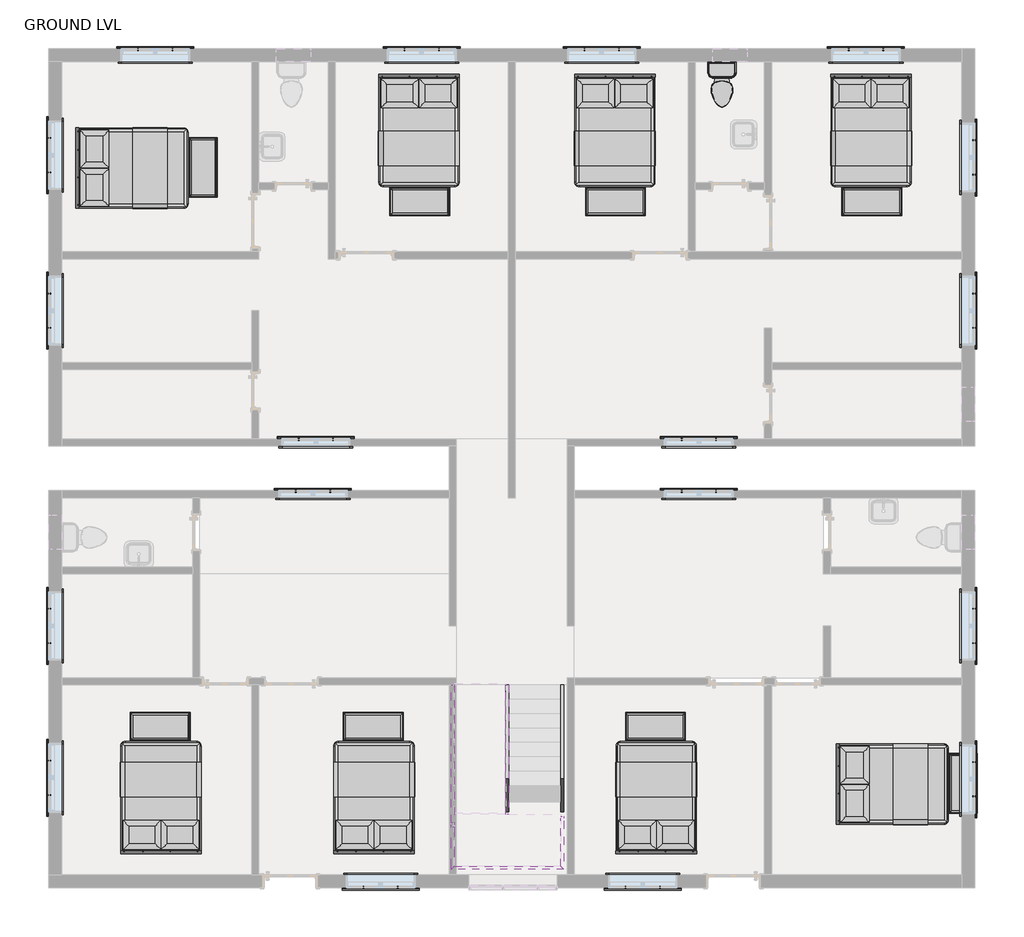
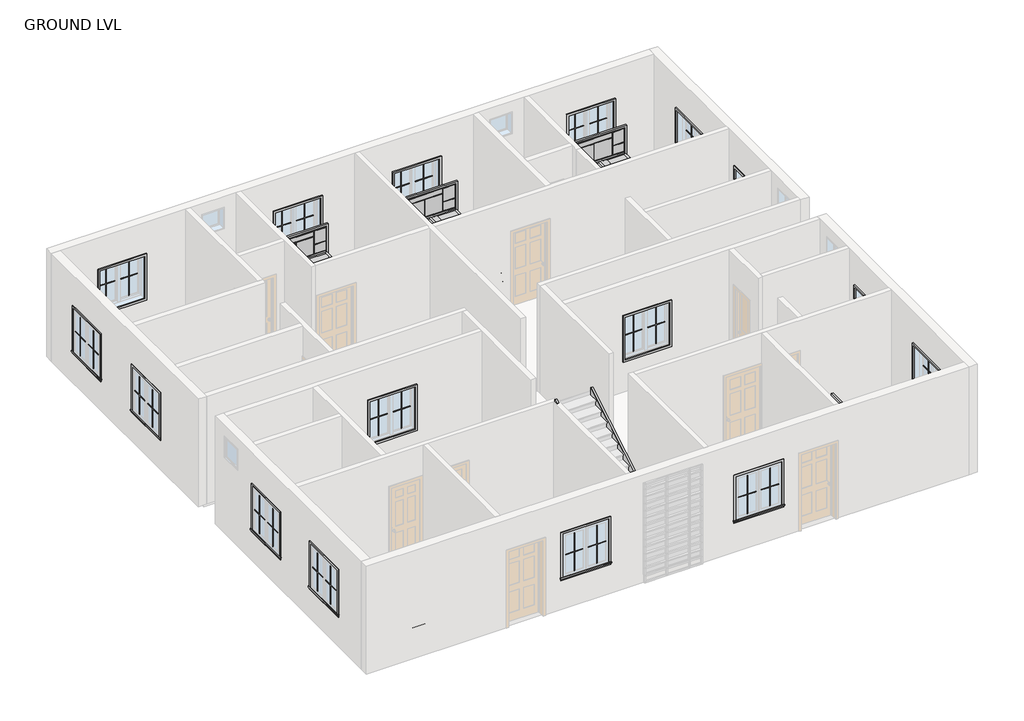
# One storey, part 4 of 4: 80 proxies, 7 members, 1 flow terminal.
"""IFC4 building model written with IfcOpenShell, lengths in millimetres."""

from ifc_helpers import new_model, si_unit, frame, origin, place, context, project, spatial, polyline, outline, extrude, faceted_brep, transform, mapped, element, save
from components import muntin_pattern_2x2_muntin_pattern_2x2_4dfeb3f3, muntin_pattern_2x2_muntin_pattern_2x2_e852a7e4, trim_window_exterior_flat_with_sill_7cfdd449, trim_window_interior_flat_picture_frame_f1e0b15b, bed_6483_bed_6483_9f93eb2d, bed_6483_bed_6483_60f1e3ed, toilet_domestic_3d_toilet_domestic_3d_ba6479b0, toilet_domestic_3d_toilet_domestic_3d_30431060

model = new_model("IFC4")

# Units and contexts
model_context = context("Model", 3, world=origin())
ifc_project = project(units=[si_unit("LENGTHUNIT", "METRE", prefix="MILLI")], contexts=[model_context])

# Site, building, storey
site = spatial("IfcSite", under=ifc_project)
building = spatial("IfcBuilding", under=site)
storey = spatial("IfcBuildingStorey", under=building, Name="GROUND LVL", Elevation=0.0)

# Proxies
placement = place(None, origin())
muntin_pattern_2x2_muntin_pattern_2x2_shape = muntin_pattern_2x2_muntin_pattern_2x2_4dfeb3f3(model_context)
element("IfcBuildingElementProxy", 1, Name="Muntin Pattern_2x2 : Muntin Pattern_2x2", ObjectType="Muntin Pattern_2x2 : Muntin Pattern_2x2", at=placement, inside=storey, context=model_context, shape_type="MappedRepresentation", body=[
    mapped(muntin_pattern_2x2_muntin_pattern_2x2_shape, transform((-12420.8887331, 2059.7281164, 984.25), x_axis=(0.0, 1.0, 0.0), y_axis=(-1.0, 0.0, 0.0), z_axis=(0.0, 0.0, 1.0))),
])
element("IfcBuildingElementProxy", 2, Name="Muntin Pattern_2x2 : Muntin Pattern_2x2", ObjectType="Muntin Pattern_2x2 : Muntin Pattern_2x2", at=placement, inside=storey, context=model_context, shape_type="MappedRepresentation", body=[
    mapped(muntin_pattern_2x2_muntin_pattern_2x2_shape, transform((-12420.8887331, 4803.7218664, 984.25), x_axis=(0.0, 1.0, 0.0), y_axis=(-1.0, 0.0, 0.0), z_axis=(0.0, 0.0, 1.0))),
])
element("IfcBuildingElementProxy", 3, Name="Muntin Pattern_2x2 : Muntin Pattern_2x2", ObjectType="Muntin Pattern_2x2 : Muntin Pattern_2x2", at=placement, inside=storey, context=model_context, shape_type="MappedRepresentation", body=[
    mapped(muntin_pattern_2x2_muntin_pattern_2x2_shape, transform((-10854.0262331, 6977.8031164, 984.25), x_axis=(1.0, 0.0, 0.0), y_axis=(0.0, 1.0, 0.0), z_axis=(0.0, 0.0, 1.0))),
])
element("IfcBuildingElementProxy", 4, Name="Muntin Pattern_2x2 : Muntin Pattern_2x2", ObjectType="Muntin Pattern_2x2 : Muntin Pattern_2x2", at=placement, inside=storey, context=model_context, shape_type="MappedRepresentation", body=[
    mapped(muntin_pattern_2x2_muntin_pattern_2x2_shape, transform((-6155.0262331, 6977.8031164, 984.25), x_axis=(1.0, 0.0, 0.0), y_axis=(0.0, 1.0, 0.0), z_axis=(0.0, 0.0, 1.0))),
])
element("IfcBuildingElementProxy", 5, Name="Muntin Pattern_2x2 : Muntin Pattern_2x2", ObjectType="Muntin Pattern_2x2 : Muntin Pattern_2x2", at=placement, inside=storey, context=model_context, shape_type="MappedRepresentation", body=[
    mapped(muntin_pattern_2x2_muntin_pattern_2x2_shape, transform((-2980.0262331, 6977.8031164, 984.25), x_axis=(1.0, 0.0, 0.0), y_axis=(0.0, 1.0, 0.0), z_axis=(0.0, 0.0, 1.0))),
])
element("IfcBuildingElementProxy", 6, Name="Muntin Pattern_2x2 : Muntin Pattern_2x2", ObjectType="Muntin Pattern_2x2 : Muntin Pattern_2x2", at=placement, inside=storey, context=model_context, shape_type="MappedRepresentation", body=[
    mapped(muntin_pattern_2x2_muntin_pattern_2x2_shape, transform((1680.8737669, 6977.8031164, 984.25), x_axis=(1.0, 0.0, 0.0), y_axis=(0.0, 1.0, 0.0), z_axis=(0.0, 0.0, 1.0))),
])
element("IfcBuildingElementProxy", 7, Name="Muntin Pattern_2x2 : Muntin Pattern_2x2", ObjectType="Muntin Pattern_2x2 : Muntin Pattern_2x2", at=placement, inside=storey, context=model_context, shape_type="MappedRepresentation", body=[
    mapped(muntin_pattern_2x2_muntin_pattern_2x2_shape, transform((3892.2612669, 5371.2531164, 984.25), x_axis=(0.0, -1.0, 0.0), y_axis=(1.0, 0.0, 0.0), z_axis=(0.0, 0.0, 1.0))),
])
element("IfcBuildingElementProxy", 8, Name="Muntin Pattern_2x2 : Muntin Pattern_2x2", ObjectType="Muntin Pattern_2x2 : Muntin Pattern_2x2", at=placement, inside=storey, context=model_context, shape_type="MappedRepresentation", body=[
    mapped(muntin_pattern_2x2_muntin_pattern_2x2_shape, transform((3892.2612669, 2666.1531164, 984.25), x_axis=(0.0, -1.0, 0.0), y_axis=(1.0, 0.0, 0.0), z_axis=(0.0, 0.0, 1.0))),
])
element("IfcBuildingElementProxy", 9, Name="Muntin Pattern_2x2 : Muntin Pattern_2x2", ObjectType="Muntin Pattern_2x2 : Muntin Pattern_2x2", at=placement, inside=storey, context=model_context, shape_type="MappedRepresentation", body=[
    mapped(muntin_pattern_2x2_muntin_pattern_2x2_shape, transform((3892.2612669, -2896.4468836, 984.25), x_axis=(0.0, -1.0, 0.0), y_axis=(1.0, 0.0, 0.0), z_axis=(0.0, 0.0, 1.0))),
])
element("IfcBuildingElementProxy", 10, Name="Muntin Pattern_2x2 : Muntin Pattern_2x2", ObjectType="Muntin Pattern_2x2 : Muntin Pattern_2x2", at=placement, inside=storey, context=model_context, shape_type="MappedRepresentation", body=[
    mapped(muntin_pattern_2x2_muntin_pattern_2x2_shape, transform((3892.2612669, -5601.5468836, 984.25), x_axis=(0.0, -1.0, 0.0), y_axis=(1.0, 0.0, 0.0), z_axis=(0.0, 0.0, 1.0))),
])
element("IfcBuildingElementProxy", 11, Name="Muntin Pattern_2x2 : Muntin Pattern_2x2", ObjectType="Muntin Pattern_2x2 : Muntin Pattern_2x2", at=placement, inside=storey, context=model_context, shape_type="MappedRepresentation", body=[
    mapped(muntin_pattern_2x2_muntin_pattern_2x2_shape, transform((-1649.7012331, -7812.9343836, 984.25), x_axis=(-1.0, 0.0, 0.0), y_axis=(0.0, -1.0, 0.0), z_axis=(0.0, 0.0, 1.0))),
])
element("IfcBuildingElementProxy", 12, Name="Muntin Pattern_2x2 : Muntin Pattern_2x2", ObjectType="Muntin Pattern_2x2 : Muntin Pattern_2x2", at=placement, inside=storey, context=model_context, shape_type="MappedRepresentation", body=[
    mapped(muntin_pattern_2x2_muntin_pattern_2x2_shape, transform((-6272.5012331, -7812.9343836, 984.25), x_axis=(-1.0, 0.0, 0.0), y_axis=(0.0, -1.0, 0.0), z_axis=(0.0, 0.0, 1.0))),
])
element("IfcBuildingElementProxy", 13, Name="Muntin Pattern_2x2 : Muntin Pattern_2x2", ObjectType="Muntin Pattern_2x2 : Muntin Pattern_2x2", at=placement, inside=storey, context=model_context, shape_type="MappedRepresentation", body=[
    mapped(muntin_pattern_2x2_muntin_pattern_2x2_shape, transform((-12420.8887331, -6182.5718836, 984.25), x_axis=(0.0, 1.0, 0.0), y_axis=(-1.0, 0.0, 0.0), z_axis=(0.0, 0.0, 1.0))),
])
element("IfcBuildingElementProxy", 14, Name="Muntin Pattern_2x2 : Muntin Pattern_2x2", ObjectType="Muntin Pattern_2x2 : Muntin Pattern_2x2", at=placement, inside=storey, context=model_context, shape_type="MappedRepresentation", body=[
    mapped(muntin_pattern_2x2_muntin_pattern_2x2_shape, transform((-12420.8887331, -3502.8718836, 984.25), x_axis=(0.0, 1.0, 0.0), y_axis=(-1.0, 0.0, 0.0), z_axis=(0.0, 0.0, 1.0))),
])
element("IfcBuildingElementProxy", 15, Name="Muntin Pattern_2x2 : Muntin Pattern_2x2", ObjectType="Muntin Pattern_2x2 : Muntin Pattern_2x2", at=placement, inside=storey, context=model_context, shape_type="MappedRepresentation", body=[
    mapped(muntin_pattern_2x2_muntin_pattern_2x2_shape, transform((-8072.7262331, -821.5843836, 984.25), x_axis=(1.0, 0.0, 0.0), y_axis=(0.0, 1.0, 0.0), z_axis=(0.0, 0.0, 1.0))),
])
element("IfcBuildingElementProxy", 16, Name="Muntin Pattern_2x2 : Muntin Pattern_2x2", ObjectType="Muntin Pattern_2x2 : Muntin Pattern_2x2", at=placement, inside=storey, context=model_context, shape_type="MappedRepresentation", body=[
    mapped(muntin_pattern_2x2_muntin_pattern_2x2_shape, transform((-8021.9262331, 92.8156164, 984.25), x_axis=(1.0, 0.0, 0.0), y_axis=(0.0, 1.0, 0.0), z_axis=(0.0, 0.0, 1.0))),
])
element("IfcBuildingElementProxy", 17, Name="Muntin Pattern_2x2 : Muntin Pattern_2x2", ObjectType="Muntin Pattern_2x2 : Muntin Pattern_2x2", at=placement, inside=storey, context=model_context, shape_type="MappedRepresentation", body=[
    mapped(muntin_pattern_2x2_muntin_pattern_2x2_shape, transform((-1265.5262331, -821.5843836, 984.25), x_axis=(1.0, 0.0, 0.0), y_axis=(0.0, 1.0, 0.0), z_axis=(0.0, 0.0, 1.0))),
])
element("IfcBuildingElementProxy", 18, Name="Muntin Pattern_2x2 : Muntin Pattern_2x2", ObjectType="Muntin Pattern_2x2 : Muntin Pattern_2x2", at=placement, inside=storey, context=model_context, shape_type="MappedRepresentation", body=[
    mapped(muntin_pattern_2x2_muntin_pattern_2x2_shape, transform((-1265.5262331, 92.8156164, 984.25), x_axis=(1.0, 0.0, 0.0), y_axis=(0.0, 1.0, 0.0), z_axis=(0.0, 0.0, 1.0))),
])
muntin_pattern_2x2_muntin_pattern_2x2_2_shape = muntin_pattern_2x2_muntin_pattern_2x2_e852a7e4(model_context)
element("IfcBuildingElementProxy", 19, Name="Muntin Pattern_2x2 : Muntin Pattern_2x2", ObjectType="Muntin Pattern_2x2 : Muntin Pattern_2x2", at=placement, inside=storey, context=model_context, shape_type="MappedRepresentation", body=[
    mapped(muntin_pattern_2x2_muntin_pattern_2x2_2_shape, transform((-12420.8887331, 2666.1531164, 984.25), x_axis=(0.0, -1.0, 0.0), y_axis=(1.0, 0.0, 0.0), z_axis=(0.0, 0.0, 1.0))),
])
element("IfcBuildingElementProxy", 20, Name="Muntin Pattern_2x2 : Muntin Pattern_2x2", ObjectType="Muntin Pattern_2x2 : Muntin Pattern_2x2", at=placement, inside=storey, context=model_context, shape_type="MappedRepresentation", body=[
    mapped(muntin_pattern_2x2_muntin_pattern_2x2_2_shape, transform((-12420.8887331, 5410.1468664, 984.25), x_axis=(0.0, -1.0, 0.0), y_axis=(1.0, 0.0, 0.0), z_axis=(0.0, 0.0, 1.0))),
])
element("IfcBuildingElementProxy", 21, Name="Muntin Pattern_2x2 : Muntin Pattern_2x2", ObjectType="Muntin Pattern_2x2 : Muntin Pattern_2x2", at=placement, inside=storey, context=model_context, shape_type="MappedRepresentation", body=[
    mapped(muntin_pattern_2x2_muntin_pattern_2x2_2_shape, transform((-10247.6012331, 6977.8031164, 984.25), x_axis=(-1.0, 0.0, 0.0), y_axis=(0.0, -1.0, 0.0), z_axis=(0.0, 0.0, 1.0))),
])
element("IfcBuildingElementProxy", 22, Name="Muntin Pattern_2x2 : Muntin Pattern_2x2", ObjectType="Muntin Pattern_2x2 : Muntin Pattern_2x2", at=placement, inside=storey, context=model_context, shape_type="MappedRepresentation", body=[
    mapped(muntin_pattern_2x2_muntin_pattern_2x2_2_shape, transform((-5548.6012331, 6977.8031164, 984.25), x_axis=(-1.0, 0.0, 0.0), y_axis=(0.0, -1.0, 0.0), z_axis=(0.0, 0.0, 1.0))),
])
element("IfcBuildingElementProxy", 23, Name="Muntin Pattern_2x2 : Muntin Pattern_2x2", ObjectType="Muntin Pattern_2x2 : Muntin Pattern_2x2", at=placement, inside=storey, context=model_context, shape_type="MappedRepresentation", body=[
    mapped(muntin_pattern_2x2_muntin_pattern_2x2_2_shape, transform((-2373.6012331, 6977.8031164, 984.25), x_axis=(-1.0, 0.0, 0.0), y_axis=(0.0, -1.0, 0.0), z_axis=(0.0, 0.0, 1.0))),
])
element("IfcBuildingElementProxy", 24, Name="Muntin Pattern_2x2 : Muntin Pattern_2x2", ObjectType="Muntin Pattern_2x2 : Muntin Pattern_2x2", at=placement, inside=storey, context=model_context, shape_type="MappedRepresentation", body=[
    mapped(muntin_pattern_2x2_muntin_pattern_2x2_2_shape, transform((2287.2987669, 6977.8031164, 984.25), x_axis=(-1.0, 0.0, 0.0), y_axis=(0.0, -1.0, 0.0), z_axis=(0.0, 0.0, 1.0))),
])
element("IfcBuildingElementProxy", 25, Name="Muntin Pattern_2x2 : Muntin Pattern_2x2", ObjectType="Muntin Pattern_2x2 : Muntin Pattern_2x2", at=placement, inside=storey, context=model_context, shape_type="MappedRepresentation", body=[
    mapped(muntin_pattern_2x2_muntin_pattern_2x2_2_shape, transform((3892.2612669, 4764.8281164, 984.25), x_axis=(0.0, 1.0, 0.0), y_axis=(-1.0, 0.0, 0.0), z_axis=(0.0, 0.0, 1.0))),
])
element("IfcBuildingElementProxy", 26, Name="Muntin Pattern_2x2 : Muntin Pattern_2x2", ObjectType="Muntin Pattern_2x2 : Muntin Pattern_2x2", at=placement, inside=storey, context=model_context, shape_type="MappedRepresentation", body=[
    mapped(muntin_pattern_2x2_muntin_pattern_2x2_2_shape, transform((3892.2612669, 2059.7281164, 984.25), x_axis=(0.0, 1.0, 0.0), y_axis=(-1.0, 0.0, 0.0), z_axis=(0.0, 0.0, 1.0))),
])
element("IfcBuildingElementProxy", 27, Name="Muntin Pattern_2x2 : Muntin Pattern_2x2", ObjectType="Muntin Pattern_2x2 : Muntin Pattern_2x2", at=placement, inside=storey, context=model_context, shape_type="MappedRepresentation", body=[
    mapped(muntin_pattern_2x2_muntin_pattern_2x2_2_shape, transform((3892.2612669, -3502.8718836, 984.25), x_axis=(0.0, 1.0, 0.0), y_axis=(-1.0, 0.0, 0.0), z_axis=(0.0, 0.0, 1.0))),
])
element("IfcBuildingElementProxy", 28, Name="Muntin Pattern_2x2 : Muntin Pattern_2x2", ObjectType="Muntin Pattern_2x2 : Muntin Pattern_2x2", at=placement, inside=storey, context=model_context, shape_type="MappedRepresentation", body=[
    mapped(muntin_pattern_2x2_muntin_pattern_2x2_2_shape, transform((3892.2612669, -6207.9718836, 984.25), x_axis=(0.0, 1.0, 0.0), y_axis=(-1.0, 0.0, 0.0), z_axis=(0.0, 0.0, 1.0))),
])
element("IfcBuildingElementProxy", 29, Name="Muntin Pattern_2x2 : Muntin Pattern_2x2", ObjectType="Muntin Pattern_2x2 : Muntin Pattern_2x2", at=placement, inside=storey, context=model_context, shape_type="MappedRepresentation", body=[
    mapped(muntin_pattern_2x2_muntin_pattern_2x2_2_shape, transform((-2256.1262331, -7812.9343836, 984.25), x_axis=(1.0, 0.0, 0.0), y_axis=(0.0, 1.0, 0.0), z_axis=(0.0, 0.0, 1.0))),
])
element("IfcBuildingElementProxy", 30, Name="Muntin Pattern_2x2 : Muntin Pattern_2x2", ObjectType="Muntin Pattern_2x2 : Muntin Pattern_2x2", at=placement, inside=storey, context=model_context, shape_type="MappedRepresentation", body=[
    mapped(muntin_pattern_2x2_muntin_pattern_2x2_2_shape, transform((-6878.9262331, -7812.9343836, 984.25), x_axis=(1.0, 0.0, 0.0), y_axis=(0.0, 1.0, 0.0), z_axis=(0.0, 0.0, 1.0))),
])
element("IfcBuildingElementProxy", 31, Name="Muntin Pattern_2x2 : Muntin Pattern_2x2", ObjectType="Muntin Pattern_2x2 : Muntin Pattern_2x2", at=placement, inside=storey, context=model_context, shape_type="MappedRepresentation", body=[
    mapped(muntin_pattern_2x2_muntin_pattern_2x2_2_shape, transform((-12420.8887331, -5576.1468836, 984.25), x_axis=(0.0, -1.0, 0.0), y_axis=(1.0, 0.0, 0.0), z_axis=(0.0, 0.0, 1.0))),
])
element("IfcBuildingElementProxy", 32, Name="Muntin Pattern_2x2 : Muntin Pattern_2x2", ObjectType="Muntin Pattern_2x2 : Muntin Pattern_2x2", at=placement, inside=storey, context=model_context, shape_type="MappedRepresentation", body=[
    mapped(muntin_pattern_2x2_muntin_pattern_2x2_2_shape, transform((-12420.8887331, -2896.4468836, 984.25), x_axis=(0.0, -1.0, 0.0), y_axis=(1.0, 0.0, 0.0), z_axis=(0.0, 0.0, 1.0))),
])
element("IfcBuildingElementProxy", 33, Name="Muntin Pattern_2x2 : Muntin Pattern_2x2", ObjectType="Muntin Pattern_2x2 : Muntin Pattern_2x2", at=placement, inside=storey, context=model_context, shape_type="MappedRepresentation", body=[
    mapped(muntin_pattern_2x2_muntin_pattern_2x2_2_shape, transform((-7466.3012331, -821.5843836, 984.25), x_axis=(-1.0, 0.0, 0.0), y_axis=(0.0, -1.0, 0.0), z_axis=(0.0, 0.0, 1.0))),
])
element("IfcBuildingElementProxy", 34, Name="Muntin Pattern_2x2 : Muntin Pattern_2x2", ObjectType="Muntin Pattern_2x2 : Muntin Pattern_2x2", at=placement, inside=storey, context=model_context, shape_type="MappedRepresentation", body=[
    mapped(muntin_pattern_2x2_muntin_pattern_2x2_2_shape, transform((-7415.5012331, 92.8156164, 984.25), x_axis=(-1.0, 0.0, 0.0), y_axis=(0.0, -1.0, 0.0), z_axis=(0.0, 0.0, 1.0))),
])
element("IfcBuildingElementProxy", 35, Name="Muntin Pattern_2x2 : Muntin Pattern_2x2", ObjectType="Muntin Pattern_2x2 : Muntin Pattern_2x2", at=placement, inside=storey, context=model_context, shape_type="MappedRepresentation", body=[
    mapped(muntin_pattern_2x2_muntin_pattern_2x2_2_shape, transform((-659.1012331, -821.5843836, 984.25), x_axis=(-1.0, 0.0, 0.0), y_axis=(0.0, -1.0, 0.0), z_axis=(0.0, 0.0, 1.0))),
])
element("IfcBuildingElementProxy", 36, Name="Muntin Pattern_2x2 : Muntin Pattern_2x2", ObjectType="Muntin Pattern_2x2 : Muntin Pattern_2x2", at=placement, inside=storey, context=model_context, shape_type="MappedRepresentation", body=[
    mapped(muntin_pattern_2x2_muntin_pattern_2x2_2_shape, transform((-659.1012331, 92.8156164, 984.25), x_axis=(-1.0, 0.0, 0.0), y_axis=(0.0, -1.0, 0.0), z_axis=(0.0, 0.0, 1.0))),
])
trim_window_exterior_flat_with_sill_shape = trim_window_exterior_flat_with_sill_7cfdd449(model_context)
element("IfcBuildingElementProxy", 37, Name="Trim-Window-Exterior-Flat : with Sill", ObjectType="Trim-Window-Exterior-Flat : with Sill", at=placement, inside=storey, context=model_context, shape_type="MappedRepresentation", body=[
    mapped(trim_window_exterior_flat_with_sill_shape, transform((-12430.4137331, 2362.9406164, 2133.6), x_axis=(0.0, -1.0, 0.0), y_axis=(0.0, 0.0, 1.0), z_axis=(-1.0, 0.0, 0.0))),
])
element("IfcBuildingElementProxy", 38, Name="Trim-Window-Exterior-Flat : with Sill", ObjectType="Trim-Window-Exterior-Flat : with Sill", at=placement, inside=storey, context=model_context, shape_type="MappedRepresentation", body=[
    mapped(trim_window_exterior_flat_with_sill_shape, transform((-12430.4137331, 5106.9343664, 2133.6), x_axis=(0.0, -1.0, 0.0), y_axis=(0.0, 0.0, 1.0), z_axis=(-1.0, 0.0, 0.0))),
])
element("IfcBuildingElementProxy", 39, Name="Trim-Window-Exterior-Flat : with Sill", ObjectType="Trim-Window-Exterior-Flat : with Sill", at=placement, inside=storey, context=model_context, shape_type="MappedRepresentation", body=[
    mapped(trim_window_exterior_flat_with_sill_shape, transform((-10550.8137331, 6987.3281164, 2133.6), x_axis=(-1.0, 0.0, 0.0), y_axis=(0.0, 0.0, 1.0), z_axis=(0.0, 1.0, 0.0))),
])
element("IfcBuildingElementProxy", 40, Name="Trim-Window-Exterior-Flat : with Sill", ObjectType="Trim-Window-Exterior-Flat : with Sill", at=placement, inside=storey, context=model_context, shape_type="MappedRepresentation", body=[
    mapped(trim_window_exterior_flat_with_sill_shape, transform((-5851.8137331, 6987.3281164, 2133.6), x_axis=(-1.0, 0.0, 0.0), y_axis=(0.0, 0.0, 1.0), z_axis=(0.0, 1.0, 0.0))),
])
element("IfcBuildingElementProxy", 41, Name="Trim-Window-Exterior-Flat : with Sill", ObjectType="Trim-Window-Exterior-Flat : with Sill", at=placement, inside=storey, context=model_context, shape_type="MappedRepresentation", body=[
    mapped(trim_window_exterior_flat_with_sill_shape, transform((-2676.8137331, 6987.3281164, 2133.6), x_axis=(-1.0, 0.0, 0.0), y_axis=(0.0, 0.0, 1.0), z_axis=(0.0, 1.0, 0.0))),
])
element("IfcBuildingElementProxy", 42, Name="Trim-Window-Exterior-Flat : with Sill", ObjectType="Trim-Window-Exterior-Flat : with Sill", at=placement, inside=storey, context=model_context, shape_type="MappedRepresentation", body=[
    mapped(trim_window_exterior_flat_with_sill_shape, transform((1984.0862669, 6987.3281164, 2133.6), x_axis=(-1.0, 0.0, 0.0), y_axis=(0.0, 0.0, 1.0), z_axis=(0.0, 1.0, 0.0))),
])
element("IfcBuildingElementProxy", 43, Name="Trim-Window-Exterior-Flat : with Sill", ObjectType="Trim-Window-Exterior-Flat : with Sill", at=placement, inside=storey, context=model_context, shape_type="MappedRepresentation", body=[
    mapped(trim_window_exterior_flat_with_sill_shape, transform((3901.7862669, 5068.0406164, 2133.6), x_axis=(0.0, 1.0, 0.0), y_axis=(0.0, 0.0, 1.0), z_axis=(1.0, 0.0, 0.0))),
])
element("IfcBuildingElementProxy", 44, Name="Trim-Window-Exterior-Flat : with Sill", ObjectType="Trim-Window-Exterior-Flat : with Sill", at=placement, inside=storey, context=model_context, shape_type="MappedRepresentation", body=[
    mapped(trim_window_exterior_flat_with_sill_shape, transform((3901.7862669, 2362.9406164, 2133.6), x_axis=(0.0, 1.0, 0.0), y_axis=(0.0, 0.0, 1.0), z_axis=(1.0, 0.0, 0.0))),
])
element("IfcBuildingElementProxy", 45, Name="Trim-Window-Exterior-Flat : with Sill", ObjectType="Trim-Window-Exterior-Flat : with Sill", at=placement, inside=storey, context=model_context, shape_type="MappedRepresentation", body=[
    mapped(trim_window_exterior_flat_with_sill_shape, transform((3901.7862669, -3199.6593836, 2133.6), x_axis=(0.0, 1.0, 0.0), y_axis=(0.0, 0.0, 1.0), z_axis=(1.0, 0.0, 0.0))),
])
element("IfcBuildingElementProxy", 46, Name="Trim-Window-Exterior-Flat : with Sill", ObjectType="Trim-Window-Exterior-Flat : with Sill", at=placement, inside=storey, context=model_context, shape_type="MappedRepresentation", body=[
    mapped(trim_window_exterior_flat_with_sill_shape, transform((3901.7862669, -5904.7593836, 2133.6), x_axis=(0.0, 1.0, 0.0), y_axis=(0.0, 0.0, 1.0), z_axis=(1.0, 0.0, 0.0))),
])
element("IfcBuildingElementProxy", 47, Name="Trim-Window-Exterior-Flat : with Sill", ObjectType="Trim-Window-Exterior-Flat : with Sill", at=placement, inside=storey, context=model_context, shape_type="MappedRepresentation", body=[
    mapped(trim_window_exterior_flat_with_sill_shape, transform((-1952.9137331, -7822.4593836, 2133.6), x_axis=(1.0, 0.0, 0.0), y_axis=(0.0, 0.0, 1.0), z_axis=(0.0, -1.0, 0.0))),
])
element("IfcBuildingElementProxy", 48, Name="Trim-Window-Exterior-Flat : with Sill", ObjectType="Trim-Window-Exterior-Flat : with Sill", at=placement, inside=storey, context=model_context, shape_type="MappedRepresentation", body=[
    mapped(trim_window_exterior_flat_with_sill_shape, transform((-6575.7137331, -7822.4593836, 2133.6), x_axis=(1.0, 0.0, 0.0), y_axis=(0.0, 0.0, 1.0), z_axis=(0.0, -1.0, 0.0))),
])
element("IfcBuildingElementProxy", 49, Name="Trim-Window-Exterior-Flat : with Sill", ObjectType="Trim-Window-Exterior-Flat : with Sill", at=placement, inside=storey, context=model_context, shape_type="MappedRepresentation", body=[
    mapped(trim_window_exterior_flat_with_sill_shape, transform((-12430.4137331, -5879.3593836, 2133.6), x_axis=(0.0, -1.0, 0.0), y_axis=(0.0, 0.0, 1.0), z_axis=(-1.0, 0.0, 0.0))),
])
element("IfcBuildingElementProxy", 50, Name="Trim-Window-Exterior-Flat : with Sill", ObjectType="Trim-Window-Exterior-Flat : with Sill", at=placement, inside=storey, context=model_context, shape_type="MappedRepresentation", body=[
    mapped(trim_window_exterior_flat_with_sill_shape, transform((-12430.4137331, -3199.6593836, 2133.6), x_axis=(0.0, -1.0, 0.0), y_axis=(0.0, 0.0, 1.0), z_axis=(-1.0, 0.0, 0.0))),
])
element("IfcBuildingElementProxy", 51, Name="Trim-Window-Exterior-Flat : with Sill", ObjectType="Trim-Window-Exterior-Flat : with Sill", at=placement, inside=storey, context=model_context, shape_type="MappedRepresentation", body=[
    mapped(trim_window_exterior_flat_with_sill_shape, transform((-7769.5137331, -812.0593836, 2133.6), x_axis=(-1.0, 0.0, 0.0), y_axis=(0.0, 0.0, 1.0), z_axis=(0.0, 1.0, 0.0))),
])
element("IfcBuildingElementProxy", 52, Name="Trim-Window-Exterior-Flat : with Sill", ObjectType="Trim-Window-Exterior-Flat : with Sill", at=placement, inside=storey, context=model_context, shape_type="MappedRepresentation", body=[
    mapped(trim_window_exterior_flat_with_sill_shape, transform((-7718.7137331, 102.3406164, 2133.6), x_axis=(-1.0, 0.0, 0.0), y_axis=(0.0, 0.0, 1.0), z_axis=(0.0, 1.0, 0.0))),
])
element("IfcBuildingElementProxy", 53, Name="Trim-Window-Exterior-Flat : with Sill", ObjectType="Trim-Window-Exterior-Flat : with Sill", at=placement, inside=storey, context=model_context, shape_type="MappedRepresentation", body=[
    mapped(trim_window_exterior_flat_with_sill_shape, transform((-962.3137331, -812.0593836, 2133.6), x_axis=(-1.0, 0.0, 0.0), y_axis=(0.0, 0.0, 1.0), z_axis=(0.0, 1.0, 0.0))),
])
element("IfcBuildingElementProxy", 54, Name="Trim-Window-Exterior-Flat : with Sill", ObjectType="Trim-Window-Exterior-Flat : with Sill", at=placement, inside=storey, context=model_context, shape_type="MappedRepresentation", body=[
    mapped(trim_window_exterior_flat_with_sill_shape, transform((-962.3137331, 102.3406164, 2133.6), x_axis=(-1.0, 0.0, 0.0), y_axis=(0.0, 0.0, 1.0), z_axis=(0.0, 1.0, 0.0))),
])
trim_window_interior_flat_picture_frame_shape = trim_window_interior_flat_picture_frame_f1e0b15b(model_context)
element("IfcBuildingElementProxy", 55, Name="Trim-Window-Interior-Flat : Picture Frame", ObjectType="Trim-Window-Interior-Flat : Picture Frame", at=placement, inside=storey, context=model_context, shape_type="MappedRepresentation", body=[
    mapped(trim_window_interior_flat_picture_frame_shape, transform((-12201.8137331, 2362.9406164, 2133.6), x_axis=(0.0, 1.0, 0.0), y_axis=(0.0, 0.0, 1.0), z_axis=(1.0, 0.0, 0.0))),
])
element("IfcBuildingElementProxy", 56, Name="Trim-Window-Interior-Flat : Picture Frame", ObjectType="Trim-Window-Interior-Flat : Picture Frame", at=placement, inside=storey, context=model_context, shape_type="MappedRepresentation", body=[
    mapped(trim_window_interior_flat_picture_frame_shape, transform((-12201.8137331, 5106.9343664, 2133.6), x_axis=(0.0, 1.0, 0.0), y_axis=(0.0, 0.0, 1.0), z_axis=(1.0, 0.0, 0.0))),
])
element("IfcBuildingElementProxy", 57, Name="Trim-Window-Interior-Flat : Picture Frame", ObjectType="Trim-Window-Interior-Flat : Picture Frame", at=placement, inside=storey, context=model_context, shape_type="MappedRepresentation", body=[
    mapped(trim_window_interior_flat_picture_frame_shape, transform((-10550.8137331, 6758.7281164, 2133.6), x_axis=(1.0, 0.0, 0.0), y_axis=(0.0, 0.0, 1.0), z_axis=(0.0, -1.0, 0.0))),
])
element("IfcBuildingElementProxy", 58, Name="Trim-Window-Interior-Flat : Picture Frame", ObjectType="Trim-Window-Interior-Flat : Picture Frame", at=placement, inside=storey, context=model_context, shape_type="MappedRepresentation", body=[
    mapped(trim_window_interior_flat_picture_frame_shape, transform((-5851.8137331, 6758.7281164, 2133.6), x_axis=(1.0, 0.0, 0.0), y_axis=(0.0, 0.0, 1.0), z_axis=(0.0, -1.0, 0.0))),
])
element("IfcBuildingElementProxy", 59, Name="Trim-Window-Interior-Flat : Picture Frame", ObjectType="Trim-Window-Interior-Flat : Picture Frame", at=placement, inside=storey, context=model_context, shape_type="MappedRepresentation", body=[
    mapped(trim_window_interior_flat_picture_frame_shape, transform((-2676.8137331, 6758.7281164, 2133.6), x_axis=(1.0, 0.0, 0.0), y_axis=(0.0, 0.0, 1.0), z_axis=(0.0, -1.0, 0.0))),
])
element("IfcBuildingElementProxy", 60, Name="Trim-Window-Interior-Flat : Picture Frame", ObjectType="Trim-Window-Interior-Flat : Picture Frame", at=placement, inside=storey, context=model_context, shape_type="MappedRepresentation", body=[
    mapped(trim_window_interior_flat_picture_frame_shape, transform((1984.0862669, 6758.7281164, 2133.6), x_axis=(1.0, 0.0, 0.0), y_axis=(0.0, 0.0, 1.0), z_axis=(0.0, -1.0, 0.0))),
])
element("IfcBuildingElementProxy", 61, Name="Trim-Window-Interior-Flat : Picture Frame", ObjectType="Trim-Window-Interior-Flat : Picture Frame", at=placement, inside=storey, context=model_context, shape_type="MappedRepresentation", body=[
    mapped(trim_window_interior_flat_picture_frame_shape, transform((3673.1862669, 5068.0406164, 2133.6), x_axis=(0.0, -1.0, 0.0), y_axis=(0.0, 0.0, 1.0), z_axis=(-1.0, 0.0, 0.0))),
])
element("IfcBuildingElementProxy", 62, Name="Trim-Window-Interior-Flat : Picture Frame", ObjectType="Trim-Window-Interior-Flat : Picture Frame", at=placement, inside=storey, context=model_context, shape_type="MappedRepresentation", body=[
    mapped(trim_window_interior_flat_picture_frame_shape, transform((3673.1862669, 2362.9406164, 2133.6), x_axis=(0.0, -1.0, 0.0), y_axis=(0.0, 0.0, 1.0), z_axis=(-1.0, 0.0, 0.0))),
])
element("IfcBuildingElementProxy", 63, Name="Trim-Window-Interior-Flat : Picture Frame", ObjectType="Trim-Window-Interior-Flat : Picture Frame", at=placement, inside=storey, context=model_context, shape_type="MappedRepresentation", body=[
    mapped(trim_window_interior_flat_picture_frame_shape, transform((3673.1862669, -3199.6593836, 2133.6), x_axis=(0.0, -1.0, 0.0), y_axis=(0.0, 0.0, 1.0), z_axis=(-1.0, 0.0, 0.0))),
])
element("IfcBuildingElementProxy", 64, Name="Trim-Window-Interior-Flat : Picture Frame", ObjectType="Trim-Window-Interior-Flat : Picture Frame", at=placement, inside=storey, context=model_context, shape_type="MappedRepresentation", body=[
    mapped(trim_window_interior_flat_picture_frame_shape, transform((3673.1862669, -5904.7593836, 2133.6), x_axis=(0.0, -1.0, 0.0), y_axis=(0.0, 0.0, 1.0), z_axis=(-1.0, 0.0, 0.0))),
])
element("IfcBuildingElementProxy", 65, Name="Trim-Window-Interior-Flat : Picture Frame", ObjectType="Trim-Window-Interior-Flat : Picture Frame", at=placement, inside=storey, context=model_context, shape_type="MappedRepresentation", body=[
    mapped(trim_window_interior_flat_picture_frame_shape, transform((-1952.9137331, -7593.8593836, 2133.6), x_axis=(-1.0, 0.0, 0.0), y_axis=(0.0, 0.0, 1.0), z_axis=(0.0, 1.0, 0.0))),
])
element("IfcBuildingElementProxy", 66, Name="Trim-Window-Interior-Flat : Picture Frame", ObjectType="Trim-Window-Interior-Flat : Picture Frame", at=placement, inside=storey, context=model_context, shape_type="MappedRepresentation", body=[
    mapped(trim_window_interior_flat_picture_frame_shape, transform((-6575.7137331, -7593.8593836, 2133.6), x_axis=(-1.0, 0.0, 0.0), y_axis=(0.0, 0.0, 1.0), z_axis=(0.0, 1.0, 0.0))),
])
element("IfcBuildingElementProxy", 67, Name="Trim-Window-Interior-Flat : Picture Frame", ObjectType="Trim-Window-Interior-Flat : Picture Frame", at=placement, inside=storey, context=model_context, shape_type="MappedRepresentation", body=[
    mapped(trim_window_interior_flat_picture_frame_shape, transform((-12201.8137331, -5879.3593836, 2133.6), x_axis=(0.0, 1.0, 0.0), y_axis=(0.0, 0.0, 1.0), z_axis=(1.0, 0.0, 0.0))),
])
element("IfcBuildingElementProxy", 68, Name="Trim-Window-Interior-Flat : Picture Frame", ObjectType="Trim-Window-Interior-Flat : Picture Frame", at=placement, inside=storey, context=model_context, shape_type="MappedRepresentation", body=[
    mapped(trim_window_interior_flat_picture_frame_shape, transform((-12201.8137331, -3199.6593836, 2133.6), x_axis=(0.0, 1.0, 0.0), y_axis=(0.0, 0.0, 1.0), z_axis=(1.0, 0.0, 0.0))),
])
element("IfcBuildingElementProxy", 69, Name="Trim-Window-Interior-Flat : Picture Frame", ObjectType="Trim-Window-Interior-Flat : Picture Frame", at=placement, inside=storey, context=model_context, shape_type="MappedRepresentation", body=[
    mapped(trim_window_interior_flat_picture_frame_shape, transform((-7769.5137331, -939.0593836, 2133.6), x_axis=(1.0, 0.0, 0.0), y_axis=(0.0, 0.0, 1.0), z_axis=(0.0, -1.0, 0.0))),
])
element("IfcBuildingElementProxy", 70, Name="Trim-Window-Interior-Flat : Picture Frame", ObjectType="Trim-Window-Interior-Flat : Picture Frame", at=placement, inside=storey, context=model_context, shape_type="MappedRepresentation", body=[
    mapped(trim_window_interior_flat_picture_frame_shape, transform((-7718.7137331, -24.6593836, 2133.6), x_axis=(1.0, 0.0, 0.0), y_axis=(0.0, 0.0, 1.0), z_axis=(0.0, -1.0, 0.0))),
])
element("IfcBuildingElementProxy", 71, Name="Trim-Window-Interior-Flat : Picture Frame", ObjectType="Trim-Window-Interior-Flat : Picture Frame", at=placement, inside=storey, context=model_context, shape_type="MappedRepresentation", body=[
    mapped(trim_window_interior_flat_picture_frame_shape, transform((-962.3137331, -939.0593836, 2133.6), x_axis=(1.0, 0.0, 0.0), y_axis=(0.0, 0.0, 1.0), z_axis=(0.0, -1.0, 0.0))),
])
element("IfcBuildingElementProxy", 72, Name="Trim-Window-Interior-Flat : Picture Frame", ObjectType="Trim-Window-Interior-Flat : Picture Frame", at=placement, inside=storey, context=model_context, shape_type="MappedRepresentation", body=[
    mapped(trim_window_interior_flat_picture_frame_shape, transform((-962.3137331, -24.6593836, 2133.6), x_axis=(1.0, 0.0, 0.0), y_axis=(0.0, 0.0, 1.0), z_axis=(0.0, -1.0, 0.0))),
])
bed_6483_bed_6483_shape = bed_6483_bed_6483_9f93eb2d(model_context)
bed_6483_bed_6483_2_shape = bed_6483_bed_6483_60f1e3ed(model_context)
element("IfcBuildingElementProxy", 73, Name="bed_6483 : bed_6483", ObjectType="bed_6483 : bed_6483", at=placement, inside=storey, context=model_context, shape_type="MappedRepresentation", body=[
    mapped(bed_6483_bed_6483_shape, transform((2212.6862669, 5474.4406164, 0.0), x_axis=(1.0, 0.0, 0.0), y_axis=(0.0, 1.0, 0.0), z_axis=(0.0, 0.0, 1.0))),
    mapped(bed_6483_bed_6483_2_shape, transform((2212.6862669, 5474.4406164, 0.0), x_axis=(1.0, 0.0, 0.0), y_axis=(0.0, 1.0, 0.0), z_axis=(0.0, 0.0, 1.0))),
])
element("IfcBuildingElementProxy", 74, Name="bed_6483 : bed_6483", ObjectType="bed_6483 : bed_6483", at=placement, inside=storey, context=model_context, shape_type="MappedRepresentation", body=[
    mapped(bed_6483_bed_6483_shape, transform((-2308.5137331, 5474.4406164, 0.0), x_axis=(1.0, 0.0, 0.0), y_axis=(0.0, 1.0, 0.0), z_axis=(0.0, 0.0, 1.0))),
    mapped(bed_6483_bed_6483_2_shape, transform((-2308.5137331, 5474.4406164, 0.0), x_axis=(1.0, 0.0, 0.0), y_axis=(0.0, 1.0, 0.0), z_axis=(0.0, 0.0, 1.0))),
])
element("IfcBuildingElementProxy", 75, Name="bed_6483 : bed_6483", ObjectType="bed_6483 : bed_6483", at=placement, inside=storey, context=model_context, shape_type="MappedRepresentation", body=[
    mapped(bed_6483_bed_6483_shape, transform((-5762.9137331, 5474.4406164, 0.0), x_axis=(1.0, 0.0, 0.0), y_axis=(0.0, 1.0, 0.0), z_axis=(0.0, 0.0, 1.0))),
    mapped(bed_6483_bed_6483_2_shape, transform((-5762.9137331, 5474.4406164, 0.0), x_axis=(1.0, 0.0, 0.0), y_axis=(0.0, 1.0, 0.0), z_axis=(0.0, 0.0, 1.0))),
])
element("IfcBuildingElementProxy", 76, Name="bed_6483 : bed_6483", ObjectType="bed_6483 : bed_6483", at=placement, inside=storey, context=model_context, shape_type="MappedRepresentation", body=[
    mapped(bed_6483_bed_6483_shape, transform((-10893.7137331, 5017.2406164, 0.0), x_axis=(0.0, 1.0, 0.0), y_axis=(-1.0, 0.0, 0.0), z_axis=(0.0, 0.0, 1.0))),
    mapped(bed_6483_bed_6483_2_shape, transform((-10893.7137331, 5017.2406164, 0.0), x_axis=(0.0, 1.0, 0.0), y_axis=(-1.0, 0.0, 0.0), z_axis=(0.0, 0.0, 1.0))),
])
element("IfcBuildingElementProxy", 77, Name="bed_6483 : bed_6483", ObjectType="bed_6483 : bed_6483", at=placement, inside=storey, context=model_context, shape_type="MappedRepresentation", body=[
    mapped(bed_6483_bed_6483_shape, transform((-6829.7137331, -6158.7593836, 0.0), x_axis=(-1.0, 0.0, 0.0), y_axis=(0.0, -1.0, 0.0), z_axis=(0.0, 0.0, 1.0))),
    mapped(bed_6483_bed_6483_2_shape, transform((-6829.7137331, -6158.7593836, 0.0), x_axis=(-1.0, 0.0, 0.0), y_axis=(0.0, -1.0, 0.0), z_axis=(0.0, 0.0, 1.0))),
])
element("IfcBuildingElementProxy", 78, Name="bed_6483 : bed_6483", ObjectType="bed_6483 : bed_6483", at=placement, inside=storey, context=model_context, shape_type="MappedRepresentation", body=[
    mapped(bed_6483_bed_6483_shape, transform((-10588.9137331, -6158.7593836, 0.0), x_axis=(-1.0, 0.0, 0.0), y_axis=(0.0, -1.0, 0.0), z_axis=(0.0, 0.0, 1.0))),
    mapped(bed_6483_bed_6483_2_shape, transform((-10588.9137331, -6158.7593836, 0.0), x_axis=(-1.0, 0.0, 0.0), y_axis=(0.0, -1.0, 0.0), z_axis=(0.0, 0.0, 1.0))),
])
element("IfcBuildingElementProxy", 79, Name="bed_6483 : bed_6483", ObjectType="bed_6483 : bed_6483", at=placement, inside=storey, context=model_context, shape_type="MappedRepresentation", body=[
    mapped(bed_6483_bed_6483_shape, transform((-1851.3137331, -6158.7593836, 0.0), x_axis=(-1.0, 0.0, 0.0), y_axis=(0.0, -1.0, 0.0), z_axis=(0.0, 0.0, 1.0))),
    mapped(bed_6483_bed_6483_2_shape, transform((-1851.3137331, -6158.7593836, 0.0), x_axis=(-1.0, 0.0, 0.0), y_axis=(0.0, -1.0, 0.0), z_axis=(0.0, 0.0, 1.0))),
])
element("IfcBuildingElementProxy", 80, Name="bed_6483 : bed_6483", ObjectType="bed_6483 : bed_6483", at=placement, inside=storey, context=model_context, shape_type="MappedRepresentation", body=[
    mapped(bed_6483_bed_6483_shape, transform((2517.4862669, -5853.9593836, 0.0), x_axis=(0.0, 1.0, 0.0), y_axis=(-1.0, 0.0, 0.0), z_axis=(0.0, 0.0, 1.0))),
    mapped(bed_6483_bed_6483_2_shape, transform((2517.4862669, -5853.9593836, 0.0), x_axis=(0.0, 1.0, 0.0), y_axis=(-1.0, 0.0, 0.0), z_axis=(0.0, 0.0, 1.0))),
])

# Flow terminal
toilet_domestic_3d_toilet_domestic_3d_shape = toilet_domestic_3d_toilet_domestic_3d_ba6479b0(model_context)
toilet_domestic_3d_toilet_domestic_3d_2_shape = toilet_domestic_3d_toilet_domestic_3d_30431060(model_context)
element("IfcFlowTerminal", 81, ObjectType="Toilet-Domestic-3D : Toilet-Domestic-3D", at=placement, inside=storey, context=model_context, shape_type="MappedRepresentation", body=[
    mapped(toilet_domestic_3d_toilet_domestic_3d_shape, transform((-555.9137331, 6264.032089, 0.0), x_axis=(1.0, 0.0, 0.0), y_axis=(0.0, 1.0, 0.0), z_axis=(0.0, 0.0, 1.0))),
    mapped(toilet_domestic_3d_toilet_domestic_3d_2_shape, transform((-555.9137331, 6264.032089, 0.0), x_axis=(1.0, 0.0, 0.0), y_axis=(0.0, 1.0, 0.0), z_axis=(0.0, 0.0, 1.0))),
])

# Members
element("IfcMember", 82, ObjectType="Stringer - 2\" Width", at=placement, inside=storey, context=model_context, shape_type="SweptSolid", body=[
    extrude(outline(polyline([(-4241.0593836, 211.5517384), (-4241.0593836, 0.0), (-4480.8978654, 0.0), (-6639.8978654, 1295.4), (-6555.4731529, 1600.2), (-4241.0593836, 211.5517384)])), frame((-3400.7137331, 0.0, 0.0), z_axis=(1.0, 0.0, 0.0), x_axis=(0.0, 1.0, 0.0)), (0.0, 0.0, 1.0), 50.8),
])
element("IfcMember", 83, ObjectType="Stringer - 2\" Width", at=placement, inside=storey, context=model_context, shape_type="SweptSolid", body=[
    extrude(outline(polyline([(-4241.0593836, 211.5517384), (-4241.0593836, 0.0), (-4480.8978654, 0.0), (-6476.2593836, 1197.2169109), (-6476.2593836, 1552.6717384), (-4241.0593836, 211.5517384)])), frame((-4365.9137331, 0.0, 0.0), z_axis=(1.0, 0.0, 0.0), x_axis=(0.0, 1.0, 0.0)), (0.0, 0.0, 1.0), 50.8),
])
element("IfcMember", 84, ObjectType="Stringer - 2\" Width", at=placement, inside=storey, context=model_context, shape_type="SweptSolid", body=[
    extrude(outline(polyline([(-6668.2209018, 1295.4), (-6752.6456143, 1600.2), (-4241.0593836, 3107.1517384), (-4241.0593836, 2751.6969109), (-6668.2209018, 1295.4)])), frame((-5331.1137331, 0.0, 0.0), z_axis=(1.0, 0.0, 0.0), x_axis=(0.0, 1.0, 0.0)), (0.0, 0.0, 1.0), 50.8),
])
element("IfcMember", 85, ObjectType="Stringer - 2\" Width", at=placement, inside=storey, context=model_context, shape_type="SweptSolid", body=[
    extrude(outline(polyline([(-6527.0593836, 1380.0969109), (-6527.0593836, 1735.5517384), (-4241.0593836, 3107.1517384), (-4241.0593836, 2751.6969109), (-6527.0593836, 1380.0969109)])), frame((-4365.9137331, 0.0, 0.0), z_axis=(1.0, 0.0, 0.0), x_axis=(0.0, 1.0, 0.0)), (0.0, 0.0, 1.0), 50.8),
])
element("IfcMember", 86, ObjectType="Stringer - 2\" Width", at=placement, inside=storey, context=model_context, shape_type="Brep", body=[
    faceted_brep([(-5280.3137331, -6752.6456143, 1600.2), (-5331.1137331, -6752.6456143, 1600.2), (-5331.1137331, -7492.2593836, 1600.2), (-5280.3137331, -7441.4593836, 1600.2), (-5280.3137331, -6668.2209018, 1295.4), (-5280.3137331, -7441.4593836, 1295.4), (-5331.1137331, -6668.2209018, 1295.4), (-5331.1137331, -7492.2593836, 1295.4)], [[[0, 1, 2, 3]], [[4, 0, 3, 5]], [[6, 4, 5, 7]], [[1, 6, 7, 2]], [[1, 0, 4, 6]], [[2, 7, 5, 3]]]),
])
element("IfcMember", 87, ObjectType="Stringer - 2\" Width", at=placement, inside=storey, context=model_context, shape_type="SweptSolid", body=[
    extrude(outline(polyline([(-5331.1137331, -7492.2593836), (-5280.3137331, -7441.4593836), (-3400.7137331, -7441.4593836), (-3349.9137331, -7492.2593836), (-5331.1137331, -7492.2593836)])), frame((0.0, 0.0, 1295.4), z_axis=(0.0, 0.0, 1.0), x_axis=(1.0, 0.0, 0.0)), (0.0, 0.0, 1.0), 304.8),
])
element("IfcMember", 88, ObjectType="Stringer - 2\" Width", at=placement, inside=storey, context=model_context, shape_type="Brep", body=[
    faceted_brep([(-3400.7137331, -7441.4593836, 1600.2), (-3349.9137331, -7492.2593836, 1600.2), (-3349.9137331, -6555.4731529, 1600.2), (-3400.7137331, -6555.4731529, 1600.2), (-3400.7137331, -7441.4593836, 1295.4), (-3400.7137331, -6639.8978654, 1295.4), (-3349.9137331, -7492.2593836, 1295.4), (-3349.9137331, -6639.8978654, 1295.4)], [[[0, 1, 2, 3]], [[4, 0, 3, 5]], [[6, 4, 5, 7]], [[1, 6, 7, 2]], [[1, 0, 4, 6]], [[2, 7, 5, 3]]]),
])

save(model, "model.ifc")

# Revit data of these elements
# Type "Muntin Pattern_2x2 : Muntin Pattern_2x2"
#   Width [instance default] = 4' - 0"
#   Thickness = 0' - 0 1/2"
#   Height [instance default] = 4' - 0"
#   Distance = 0' - 0 3/4"
#   Interior Material [instance default] = none
#   Exterior Material [instance default] = none
#   Default Elevation = 0
# Type "Trim-Window-Exterior-Flat : with Sill"
#   Trim Width = 0' - 2 1/4"
#   Trim Thickness_Picture Frame = 0' - 1 1/4"
#   Trim Thickness_with Sill = 0' - 0 3/4"
#   Sill Thickness = 0' - 1 1/4"
#   Opening Width [instance default] = 2' - 0"
#   Opening Height [instance default] = 3' - 0"
#   Default Elevation = 4' - 0"
#   Sill = yes
#   Picture Frame = no
#   Trim Material [instance default] = none
# Type "Trim-Window-Interior-Flat : Picture Frame"
#   Trim Thickness_Picture Frame = 0' - 1 1/4"
#   Trim Width = 0' - 2 1/4"
#   Trim Thickness_with Sill = 0' - 0 3/4"
#   Sill Thickness = 0' - 1 1/4"
#   Opening Width [instance default] = 2' - 0"
#   Opening Height [instance default] = 3' - 0"
#   Default Elevation = 4' - 0"
#   Sill = no
#   Picture Frame = yes
#   Trim Material [instance default] = none
# Type "bed_6483 : bed_6483"
#   wood = none
#   fabric 2 [instance default] = none
#   fabric [instance default] = none
#   Mirror = none
#   Default Elevation = 0
# Type "Toilet-Domestic-3D : Toilet-Domestic-3D"
#   Assembly Code = "D2010110"
#   Toilet - Bowl/Basin Material = Porcelain, Linen
#   Toilet - Seat Material = Laminate, Linen, Matte
#   Default Elevation = 0
# Elements 1, 2, 3, 4, 5, 6, 7, 8, 9, 10, 11, 12, 13, 14, 15, 16, 17, 18, 19, 20, 21, 22, 23, 24, 25, 26, 27, 28, 29, 30, 31, 32, 33, 34, 35, 36 (IfcBuildingElementProxy, "Muntin Pattern_2x2 : Muntin Pattern_2x2")
#   Width = 1' - 6 5/8"
#   Height = 3' - 6 1/2"
#   Interior Material = Wood - Stained
#   Exterior Material = Clad - White
#   Phase Created = New Construction
#   Materials on its faces: "Clad - White", "Wood - Stained"
# Elements 37, 38, 39, 40, 41, 42, 43, 44, 45, 46, 47, 48, 49, 50, 51, 52, 53, 54 (IfcBuildingElementProxy, "Trim-Window-Exterior-Flat : with Sill")
#   Opening Width = 4' - 0"
#   Opening Height = 4' - 0"
#   Trim Material = Clad - White
#   Phase Created = New Construction
#   Materials on its faces: "Clad - White"
# Elements 55, 56, 57, 58, 59, 60, 61, 62, 63, 64, 65, 66, 67, 68, 69, 70, 71, 72 (IfcBuildingElementProxy, "Trim-Window-Interior-Flat : Picture Frame")
#   Opening Width = 4' - 0"
#   Opening Height = 4' - 0"
#   Trim Material = Wood - Stained
#   Phase Created = New Construction
#   Materials on its faces: "Wood - Stained"
# Elements 73, 74, 75, 76, 77, 78, 79, 80 (IfcBuildingElementProxy, "bed_6483 : bed_6483")
#   fabric 2 = none
#   fabric = none
#   Phase Created = New Construction
#   Materials on its faces: "wood", "fabric", "fabric 2", "mirror", "chrome"
# Element 81 (IfcFlowTerminal, "Toilet-Domestic-3D : Toilet-Domestic-3D")
#   Mark = "2"
#   Phase Created = New Construction
#   Materials on its faces: "Porcelain, Linen", "Laminate, Linen, Matte"
# Elements 82, 83, 84, 85, 86, 87, 88 (IfcMember, "Stringer - 2\" Width")
#   Phase Created = New Construction
# Materials
#   "Porcelain, Linen": class "Ceramic", colour RGB 249 239 230, transparency 0, Description = "Porcelain, linen", Cost = 0
#   "Laminate, Linen, Matte": class "Plastic", colour RGB 249 239 230, transparency 0, Description = "Plastic Laminate - Linen, Matte", Cost = 0
#   "Clad - White": class "Wood", colour RGB 242 242 238, transparency 0, Cost = 0
#   "Wood - Stained": class "Wood", colour RGB 224 178 126, transparency 0, Cost = 0
#   "wood": class "Wood", colour RGB 71 38 7, transparency 0
#   "fabric": class "Fabric", colour RGB 56 56 56, transparency 0
#   "fabric 2": class "Fabric", colour RGB 64 0 0, transparency 0
#   "mirror": class "Glass", colour RGB 228 228 228, transparency 0.06
#   "chrome": class "Metal", colour RGB 244 244 244, transparency 0
